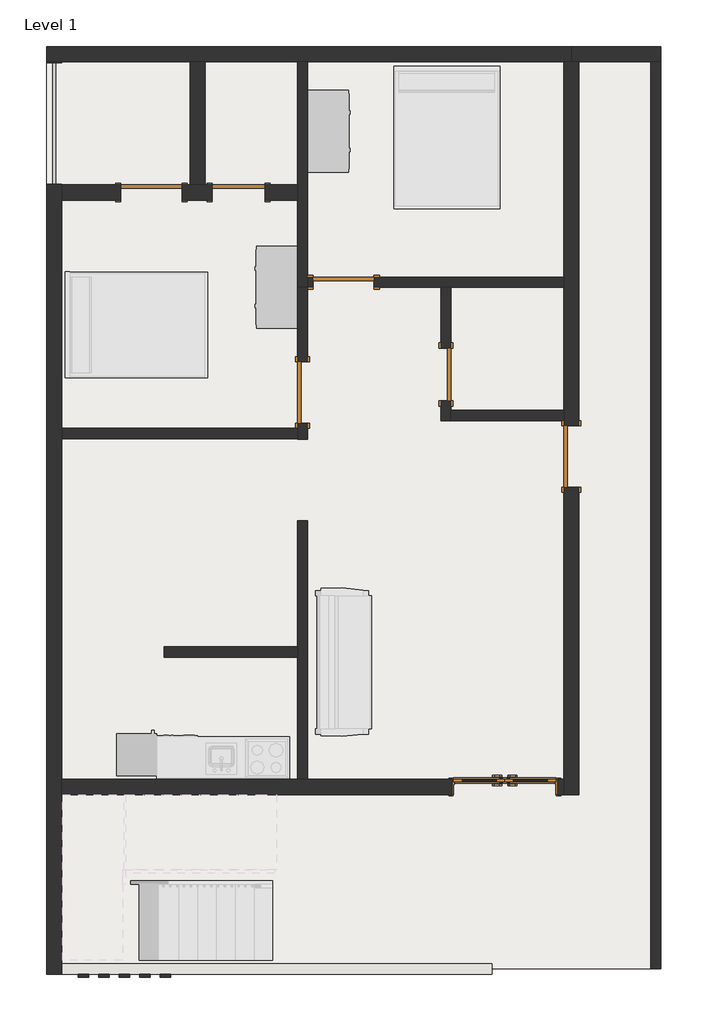
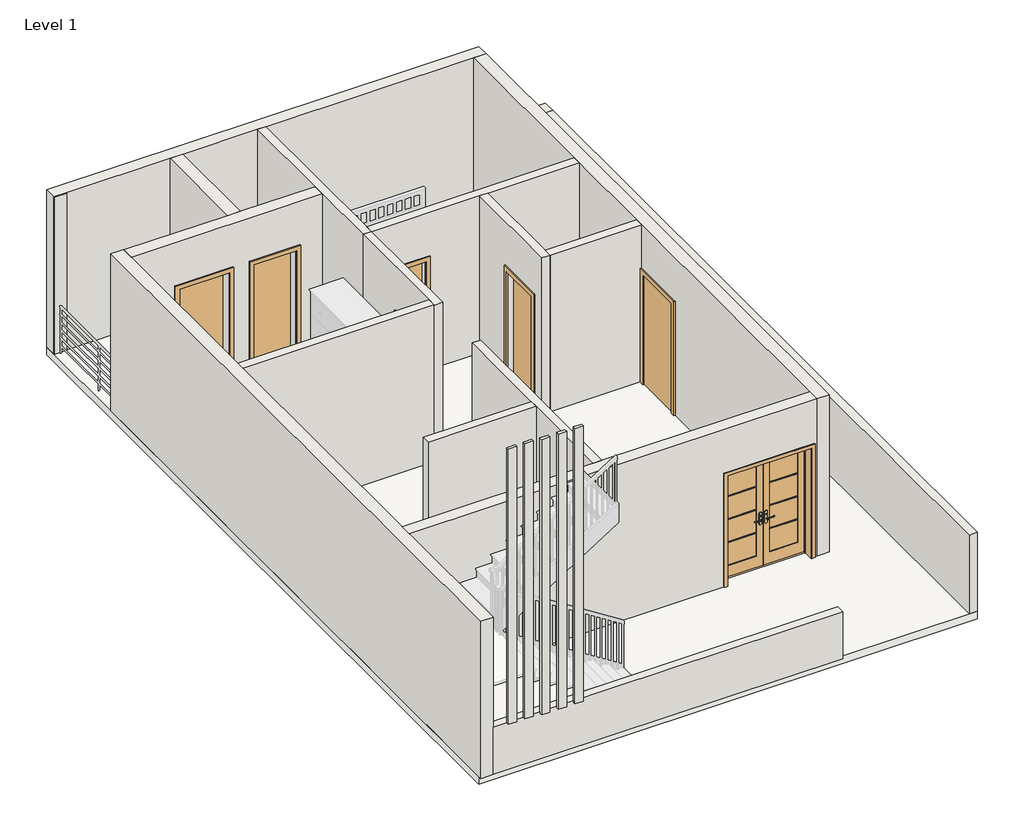
# One storey, part 1 of 2: 19 walls, 7 doors, 1 slab.
"""IFC4 building model written with IfcOpenShell, lengths in millimetres."""

from ifc_helpers import new_model, si_unit, frame, origin, origin_with_axes, place, context, project, spatial, polyline, outline, extrude, faceted_brep, transform, mapped, element, save
from components import door_014e9f54, door_486760f8, door_b804d09e, door_686f89d2, door_0ca8825f, walls_1_walls_1_4968a21e

model = new_model("IFC4")

# Units and contexts
model_context = context("Model", 3, world=origin())
ifc_project = project(units=[si_unit("LENGTHUNIT", "METRE", prefix="MILLI")], contexts=[model_context])

# Site, building, storey
site = spatial("IfcSite", under=ifc_project)
building = spatial("IfcBuilding", under=site)
storey = spatial("IfcBuildingStorey", under=building, Name="Level 1", Elevation=0.0)

# Doors
placement = place(None, origin())
door_shape = door_014e9f54(model_context)
element("IfcDoor", 1, ObjectType="Door-Exterior-Double-Full Glass-Wood_Clad : 60\" x 84\"", at=placement, inside=storey, context=model_context, shape_type="MappedRepresentation", body=[
    mapped(door_shape, transform((-4531.8683044, -1257.1141189, 0.0), x_axis=(1.0, 0.0, 0.0), y_axis=(0.0, 1.0, 0.0), z_axis=(0.0, 0.0, 1.0))),
])
door_2_shape = door_486760f8(model_context)
element("IfcDoor", 2, ObjectType="Single-Flush : 2'7\"", at=placement, inside=storey, context=model_context, shape_type="MappedRepresentation", body=[
    mapped(door_2_shape, transform((-8494.2683044, 7578.9108811, 0.0), x_axis=(-1.0, 0.0, 0.0), y_axis=(0.0, -1.0, 0.0), z_axis=(0.0, 0.0, 1.0))),
])
door_3_shape = door_b804d09e(model_context)
element("IfcDoor", 3, ObjectType="Single-Flush : 2'7\"", at=placement, inside=storey, context=model_context, shape_type="MappedRepresentation", body=[
    mapped(door_3_shape, transform((-5408.1683044, 4873.8108811, 0.0), x_axis=(0.0, -1.0, 0.0), y_axis=(1.0, 0.0, 0.0), z_axis=(0.0, 0.0, 1.0))),
])
door_4_shape = door_686f89d2(model_context)
element("IfcDoor", 4, ObjectType="Single-Flush : 36\" x 84\"", at=placement, inside=storey, context=model_context, shape_type="MappedRepresentation", body=[
    mapped(door_4_shape, transform((-6932.1683044, 6245.4108811, 0.0), x_axis=(-1.0, 0.0, 0.0), y_axis=(0.0, -1.0, 0.0), z_axis=(0.0, 0.0, 1.0))),
])
element("IfcDoor", 5, ObjectType="Single-Flush : 36\" x 84\"", at=placement, inside=storey, context=model_context, shape_type="MappedRepresentation", body=[
    mapped(door_4_shape, transform((-7541.7683044, 4607.1108811, 0.0), x_axis=(0.0, -1.0, 0.0), y_axis=(1.0, 0.0, 0.0), z_axis=(0.0, 0.0, 1.0))),
])
door_5_shape = door_0ca8825f(model_context)
element("IfcDoor", 6, ObjectType="Single-Flush : 36\" x 84\"", at=placement, inside=storey, context=model_context, shape_type="MappedRepresentation", body=[
    mapped(door_5_shape, transform((-9789.6683044, 7578.9108811, 0.0), x_axis=(1.0, 0.0, 0.0), y_axis=(0.0, 1.0, 0.0), z_axis=(0.0, 0.0, 1.0))),
])
element("IfcDoor", 7, ObjectType="Single-Flush : 36\" x 84\"", at=placement, inside=storey, context=model_context, shape_type="MappedRepresentation", body=[
    mapped(door_5_shape, transform((-3541.2683044, 3654.6108811, 0.0), x_axis=(0.0, 1.0, 0.0), y_axis=(-1.0, 0.0, 0.0), z_axis=(0.0, 0.0, 1.0))),
])

# Slab
element("IfcSlab", 8, ObjectType="6\"", at=placement, inside=storey, context=model_context, shape_type="SweptSolid", body=[
    extrude(outline(polyline([(-2207.7683044, 9750.6108811), (-2207.7683044, -3965.3891189), (-11351.7683044, -3965.3891189), (-11351.7683044, 9750.6108811), (-2207.7683044, 9750.6108811)])), frame((0.0, 0.0, -152.4), z_axis=(0.0, 0.0, 1.0), x_axis=(1.0, 0.0, 0.0)), (0.0, 0.0, 1.0), 152.4),
])

# Walls
element("IfcWall", 9, ObjectType="6\"", at=placement, inside=storey, context=model_context, shape_type="SweptSolid", body=[
    extrude(outline(polyline([(-2360.1683044, -3965.3891189), (-2360.1683044, 9522.0108811), (-2207.7683044, 9522.0108811), (-2207.7683044, -3965.3891189), (-2360.1683044, -3965.3891189)])), origin_with_axes(), (0.0, 0.0, 1.0), 1524.0),
])
element("IfcWall", 10, ObjectType="6\"", at=placement, inside=storey, context=model_context, shape_type="SweptSolid", body=[
    extrude(outline(polyline([(-11123.1683044, -3889.1891189), (-4722.3683044, -3889.1891189), (-4722.3683044, -4041.5891189), (-11123.1683044, -4041.5891189), (-11123.1683044, -3889.1891189)])), origin_with_axes(), (0.0, 0.0, 1.0), 914.4),
])
element("IfcWall", 11, ObjectType="6\" 2", at=placement, inside=storey, context=model_context, shape_type="Brep", body=[
    faceted_brep([(-7617.9683044, 9522.0108811, 0.0), (-7617.9683044, 7693.2108811, 0.0), (-7617.9683044, 7464.6108811, 0.0), (-7617.9683044, 6169.2108811, 0.0), (-7617.9683044, 6169.2108811, 3048.0), (-7617.9683044, 7464.6108811, 3048.0), (-7617.9683044, 7693.2108811, 3048.0), (-7617.9683044, 9522.0108811, 3048.0), (-7465.5683044, 9522.0108811, 0.0), (-7465.5683044, 9522.0108811, 3048.0), (-7465.5683044, 6321.6108811, 3048.0), (-7465.5683044, 6169.2108811, 3048.0), (-7465.5683044, 6169.2108811, 0.0), (-7465.5683044, 6321.6108811, 0.0)], [[[0, 1, 2, 3, 4, 5, 6, 7]], [[8, 9, 10, 11, 12, 13]], [[3, 2, 1, 0, 8, 13, 12]], [[7, 6, 5, 4, 11, 10, 9]], [[0, 7, 9, 8]], [[4, 3, 12, 11]]]),
])
element("IfcWall", 12, ObjectType="6\" 2", at=placement, inside=storey, context=model_context, shape_type="Brep", body=[
    faceted_brep([(-7465.5683044, 6169.2108811, 0.0), (-7389.3683044, 6169.2108811, 0.0), (-7389.3683044, 6169.2108811, 2133.6), (-6474.9683044, 6169.2108811, 2133.6), (-6474.9683044, 6169.2108811, 0.0), (-5484.3683044, 6169.2108811, 0.0), (-5331.9683044, 6169.2108811, 0.0), (-3655.5683044, 6169.2108811, 0.0), (-3655.5683044, 6169.2108811, 3048.0), (-5331.9683044, 6169.2108811, 3048.0), (-5484.3683044, 6169.2108811, 3048.0), (-7465.5683044, 6169.2108811, 3048.0), (-7389.3683044, 6321.6108811, 2133.6), (-7389.3683044, 6321.6108811, 0.0), (-7465.5683044, 6321.6108811, 0.0), (-7465.5683044, 6321.6108811, 3048.0), (-3655.5683044, 6321.6108811, 3048.0), (-3655.5683044, 6321.6108811, 0.0), (-6474.9683044, 6321.6108811, 0.0), (-6474.9683044, 6321.6108811, 2133.6)], [[[0, 1, 2, 3, 4, 5, 6, 7, 8, 9, 10, 11]], [[12, 13, 14, 15, 16, 17, 18, 19]], [[18, 17, 7, 6, 5, 4]], [[14, 13, 1, 0]], [[11, 10, 9, 8, 16, 15]], [[0, 11, 15, 14]], [[8, 7, 17, 16]], [[2, 1, 13, 12]], [[3, 2, 12, 19]], [[4, 3, 19, 18]]]),
])
element("IfcWall", 13, ObjectType="6\" 2", at=placement, inside=storey, context=model_context, shape_type="Brep", body=[
    faceted_brep([(-7617.9683044, 4149.9108811, 2133.6), (-7617.9683044, 4149.9108811, 0.0), (-7617.9683044, 4073.7108811, 0.0), (-7617.9683044, 3921.3108811, 0.0), (-7617.9683044, 3908.6108811, 0.0), (-7617.9683044, 3908.6108811, 3048.0), (-7617.9683044, 3921.3108811, 3048.0), (-7617.9683044, 4073.7108811, 3048.0), (-7617.9683044, 6169.2108811, 3048.0), (-7617.9683044, 6169.2108811, 0.0), (-7617.9683044, 5064.3108811, 0.0), (-7617.9683044, 5064.3108811, 2133.6), (-7465.5683044, 3908.6108811, 0.0), (-7465.5683044, 4149.9108811, 0.0), (-7465.5683044, 4149.9108811, 2133.6), (-7465.5683044, 5064.3108811, 2133.6), (-7465.5683044, 5064.3108811, 0.0), (-7465.5683044, 6169.2108811, 0.0), (-7465.5683044, 6169.2108811, 3048.0), (-7465.5683044, 3908.6108811, 3048.0)], [[[0, 1, 2, 3, 4, 5, 6, 7, 8, 9, 10, 11]], [[12, 13, 14, 15, 16, 17, 18, 19]], [[10, 9, 17, 16]], [[4, 3, 2, 1, 13, 12]], [[5, 4, 12, 19]], [[8, 7, 6, 5, 19, 18]], [[9, 8, 18, 17]], [[14, 13, 1, 0]], [[15, 14, 0, 11]], [[16, 15, 11, 10]]]),
])
element("IfcWall", 14, ObjectType="6\" 2", at=placement, inside=storey, context=model_context, shape_type="SweptSolid", body=[
    extrude(outline(polyline([(-7617.9683044, 3921.3108811), (-11123.1683044, 3921.3108811), (-11123.1683044, 4073.7108811), (-7617.9683044, 4073.7108811), (-7617.9683044, 3921.3108811)])), origin_with_axes(), (0.0, 0.0, 1.0), 3048.0),
])
element("IfcWall", 15, ObjectType="6\" 2", at=placement, inside=storey, context=model_context, shape_type="SweptSolid", body=[
    extrude(outline(polyline([(-9599.1683044, 822.5108811), (-7617.9683044, 822.5108811), (-7617.9683044, 670.1108811), (-9599.1683044, 670.1108811), (-9599.1683044, 822.5108811)])), origin_with_axes(), (0.0, 0.0, 1.0), 3048.0),
])
element("IfcWall", 16, ObjectType="6\" 2", at=placement, inside=storey, context=model_context, shape_type="Brep", body=[
    faceted_brep([(-5484.3683044, 4480.1108811, 2133.6), (-5484.3683044, 4480.1108811, 0.0), (-5484.3683044, 4188.0108811, 0.0), (-5484.3683044, 4188.0108811, 3048.0), (-5484.3683044, 6169.2108811, 3048.0), (-5484.3683044, 6169.2108811, 0.0), (-5484.3683044, 5267.5108811, 0.0), (-5484.3683044, 5267.5108811, 2133.6), (-5331.9683044, 4188.0108811, 0.0), (-5331.9683044, 4480.1108811, 0.0), (-5331.9683044, 4480.1108811, 2133.6), (-5331.9683044, 5267.5108811, 2133.6), (-5331.9683044, 5267.5108811, 0.0), (-5331.9683044, 6169.2108811, 0.0), (-5331.9683044, 6169.2108811, 3048.0), (-5331.9683044, 4340.4108811, 3048.0), (-5331.9683044, 4188.0108811, 3048.0), (-5331.9683044, 4188.0108811, 13.8133607)], [[[0, 1, 2, 3, 4, 5, 6, 7]], [[8, 9, 10, 11, 12, 13, 14, 15, 16, 17]], [[6, 5, 13, 12]], [[2, 1, 9, 8]], [[4, 3, 16, 15, 14]], [[5, 4, 14, 13]], [[3, 2, 8, 17, 16]], [[10, 9, 1, 0]], [[11, 10, 0, 7]], [[12, 11, 7, 6]]]),
])
element("IfcWall", 17, ObjectType="6\" 2", at=placement, inside=storey, context=model_context, shape_type="SweptSolid", body=[
    extrude(outline(polyline([(-3655.5683044, 4188.0108811), (-5331.9683044, 4188.0108811), (-5331.9683044, 4340.4108811), (-3655.5683044, 4340.4108811), (-3655.5683044, 4188.0108811)])), frame((0.0, 0.0, 13.8133607), z_axis=(0.0, 0.0, 1.0), x_axis=(1.0, 0.0, 0.0)), (0.0, 0.0, 1.0), 3034.1866393),
])
element("IfcWall", 18, ObjectType="6\" 2", at=placement, inside=storey, context=model_context, shape_type="Brep", body=[
    faceted_brep([(-7617.9683044, 2702.1108811, 0.0), (-7617.9683044, 822.5108811, 0.0), (-7617.9683044, 670.1108811, 0.0), (-7617.9683044, -1145.9891189, 0.0), (-7617.9683044, -1145.9891189, 3048.0), (-7617.9683044, 670.1108811, 3048.0), (-7617.9683044, 822.5108811, 3048.0), (-7617.9683044, 2702.1108811, 3048.0), (-7465.5683044, 2702.1108811, 0.0), (-7465.5683044, 2702.1108811, 3048.0), (-7465.5683044, -1145.9891189, 3048.0), (-7465.5683044, -1145.9891189, 0.0)], [[[0, 1, 2, 3, 4, 5, 6, 7]], [[8, 9, 10, 11]], [[3, 2, 1, 0, 8, 11]], [[7, 6, 5, 4, 10, 9]], [[0, 7, 9, 8]], [[4, 3, 11, 10]]]),
])
element("IfcWall", 19, ObjectType="9\"", at=placement, inside=storey, context=model_context, shape_type="Brep", body=[
    faceted_brep([(-11351.7683044, 9522.0108811, 0.0), (-11123.1683044, 9522.0108811, 0.0), (-9218.1683044, 9522.0108811, 0.0), (-8989.5683044, 9522.0108811, 0.0), (-7617.9683044, 9522.0108811, 0.0), (-7465.5683044, 9522.0108811, 0.0), (-3655.5683044, 9522.0108811, 0.0), (-3541.2683044, 9522.0108811, 0.0), (-3541.2683044, 9522.0108811, 1524.0), (-3426.9683044, 9522.0108811, 1524.0), (-3426.9683044, 9522.0108811, 3048.0), (-3655.5683044, 9522.0108811, 3048.0), (-7465.5683044, 9522.0108811, 3048.0), (-7617.9683044, 9522.0108811, 3048.0), (-8989.5683044, 9522.0108811, 3048.0), (-9218.1683044, 9522.0108811, 3048.0), (-11123.1683044, 9522.0108811, 3048.0), (-11351.7683044, 9522.0108811, 3048.0), (-11351.7683044, 9750.6108811, 0.0), (-11351.7683044, 9750.6108811, 3048.0), (-3426.9683044, 9750.6108811, 3048.0), (-3426.9683044, 9750.6108811, 1524.0), (-3541.2683044, 9750.6108811, 1524.0), (-3541.2683044, 9750.6108811, 0.0)], [[[0, 1, 2, 3, 4, 5, 6, 7, 8, 9, 10, 11, 12, 13, 14, 15, 16, 17]], [[18, 19, 20, 21, 22, 23]], [[7, 6, 5, 4, 3, 2, 1, 0, 18, 23]], [[17, 16, 15, 14, 13, 12, 11, 10, 20, 19]], [[0, 17, 19, 18]], [[8, 7, 23, 22]], [[21, 9, 8, 22]], [[10, 9, 21, 20]]]),
])
element("IfcWall", 20, ObjectType="9\"", at=placement, inside=storey, context=model_context, shape_type="Brep", body=[
    faceted_brep([(-11123.1683044, -4041.5891189, 0.0), (-11123.1683044, -3889.1891189, 0.0), (-11123.1683044, -1374.5891189, 0.0), (-11123.1683044, -1145.9891189, 0.0), (-11123.1683044, 3921.3108811, 0.0), (-11123.1683044, 4073.7108811, 0.0), (-11123.1683044, 7464.6108811, 0.0), (-11123.1683044, 7693.2108811, 0.0), (-11123.1683044, 7705.9108811, 0.0), (-11123.1683044, 7705.9108811, 3048.0), (-11123.1683044, 7693.2108811, 3048.0), (-11123.1683044, 7464.6108811, 3048.0), (-11123.1683044, 4073.7108811, 3048.0), (-11123.1683044, 3921.3108811, 3048.0), (-11123.1683044, -1145.9891189, 3048.0), (-11123.1683044, -1374.5891189, 3048.0), (-11123.1683044, -4041.5891189, 3048.0), (-11123.1683044, -4041.5891189, 914.4), (-11351.7683044, -4041.5891189, 0.0), (-11351.7683044, -4041.5891189, 3048.0), (-11351.7683044, 7705.9108811, 3048.0), (-11351.7683044, 7705.9108811, 0.0)], [[[0, 1, 2, 3, 4, 5, 6, 7, 8, 9, 10, 11, 12, 13, 14, 15, 16, 17]], [[18, 19, 20, 21]], [[8, 7, 6, 5, 4, 3, 2, 1, 0, 18, 21]], [[9, 8, 21, 20]], [[16, 15, 14, 13, 12, 11, 10, 9, 20, 19]], [[0, 17, 16, 19, 18]]]),
])
element("IfcWall", 21, ObjectType="9\"", at=placement, inside=storey, context=model_context, shape_type="Brep", body=[
    faceted_brep([(-3655.5683044, -1374.5891189, 3048.0), (-3655.5683044, -1145.9891189, 3048.0), (-3655.5683044, 4188.0108811, 3048.0), (-3655.5683044, 4340.4108811, 3048.0), (-3655.5683044, 6169.2108811, 3048.0), (-3655.5683044, 6321.6108811, 3048.0), (-3655.5683044, 9522.0108811, 3048.0), (-3655.5683044, 9522.0108811, 0.0), (-3655.5683044, 6321.6108811, 0.0), (-3655.5683044, 6169.2108811, 0.0), (-3655.5683044, 4111.8108811, 0.0), (-3655.5683044, 4111.8108811, 2133.6), (-3655.5683044, 3197.4108811, 2133.6), (-3655.5683044, 3197.4108811, 0.0), (-3655.5683044, -1145.9891189, 0.0), (-3655.5683044, -1374.5891189, 0.0), (-3426.9683044, 9522.0108811, 3048.0), (-3426.9683044, -1374.5891189, 3048.0), (-3426.9683044, -1374.5891189, 0.0), (-3426.9683044, 3197.4108811, 0.0), (-3426.9683044, 3197.4108811, 2133.6), (-3426.9683044, 4111.8108811, 2133.6), (-3426.9683044, 4111.8108811, 0.0), (-3426.9683044, 9522.0108811, 0.0), (-3426.9683044, 9522.0108811, 1524.0), (-3541.2683044, 9522.0108811, 0.0)], [[[0, 1, 2, 3, 4, 5, 6, 7, 8, 9, 10, 11, 12, 13, 14, 15]], [[16, 17, 18, 19, 20, 21, 22, 23, 24]], [[18, 15, 14, 13, 19]], [[7, 25, 23, 22, 10, 9, 8]], [[6, 5, 4, 3, 2, 1, 0, 17, 16]], [[0, 15, 18, 17]], [[23, 25, 7, 6, 16, 24]], [[21, 11, 10, 22]], [[11, 21, 20, 12]], [[12, 20, 19, 13]]]),
])
element("IfcWall", 22, ObjectType="9\"", at=placement, inside=storey, context=model_context, shape_type="Brep", body=[
    faceted_brep([(-11123.1683044, -1145.9891189, 3048.0), (-7617.9683044, -1145.9891189, 3048.0), (-7465.5683044, -1145.9891189, 3048.0), (-3655.5683044, -1145.9891189, 3048.0), (-3655.5683044, -1145.9891189, 0.0), (-3744.4683044, -1145.9891189, 0.0), (-3744.4683044, -1145.9891189, 2159.0), (-5319.2683044, -1145.9891189, 2159.0), (-5319.2683044, -1145.9891189, 0.0), (-7465.5683044, -1145.9891189, 0.0), (-7617.9683044, -1145.9891189, 0.0), (-11123.1683044, -1145.9891189, 0.0), (-3655.5683044, -1374.5891189, 3048.0), (-11123.1683044, -1374.5891189, 3048.0), (-11123.1683044, -1374.5891189, 0.0), (-5319.2683044, -1374.5891189, 0.0), (-5319.2683044, -1374.5891189, 2159.0), (-3744.4683044, -1374.5891189, 2159.0), (-3744.4683044, -1374.5891189, 0.0), (-3655.5683044, -1374.5891189, 0.0)], [[[0, 1, 2, 3, 4, 5, 6, 7, 8, 9, 10, 11]], [[12, 13, 14, 15, 16, 17, 18, 19]], [[4, 19, 18, 5]], [[14, 11, 10, 9, 8, 15]], [[3, 2, 1, 0, 13, 12]], [[4, 3, 12, 19]], [[0, 11, 14, 13]], [[17, 6, 5, 18]], [[6, 17, 16, 7]], [[7, 16, 15, 8]]]),
])
element("IfcWall", 23, ObjectType="9\"", at=placement, inside=storey, context=model_context, shape_type="Brep", body=[
    faceted_brep([(-9332.4683044, 7464.6108811, 0.0), (-8887.9683044, 7464.6108811, 0.0), (-8887.9683044, 7464.6108811, 2133.6), (-8100.5683044, 7464.6108811, 2133.6), (-8100.5683044, 7464.6108811, 0.0), (-7617.9683044, 7464.6108811, 0.0), (-7617.9683044, 7464.6108811, 3048.0), (-11123.1683044, 7464.6108811, 3048.0), (-11123.1683044, 7464.6108811, 0.0), (-10246.8683044, 7464.6108811, 0.0), (-10246.8683044, 7464.6108811, 2133.6), (-9332.4683044, 7464.6108811, 2133.6), (-8887.9683044, 7693.2108811, 2133.6), (-8887.9683044, 7693.2108811, 0.0), (-8989.5683044, 7693.2108811, 0.0), (-9218.1683044, 7693.2108811, 0.0), (-9332.4683044, 7693.2108811, 0.0), (-9332.4683044, 7693.2108811, 2133.6), (-10246.8683044, 7693.2108811, 2133.6), (-10246.8683044, 7693.2108811, 0.0), (-11123.1683044, 7693.2108811, 0.0), (-11123.1683044, 7693.2108811, 3048.0), (-9218.1683044, 7693.2108811, 3048.0), (-8989.5683044, 7693.2108811, 3048.0), (-7617.9683044, 7693.2108811, 3048.0), (-7617.9683044, 7693.2108811, 0.0), (-8100.5683044, 7693.2108811, 0.0), (-8100.5683044, 7693.2108811, 2133.6)], [[[0, 1, 2, 3, 4, 5, 6, 7, 8, 9, 10, 11]], [[12, 13, 14, 15, 16, 17, 18, 19, 20, 21, 22, 23, 24, 25, 26, 27]], [[9, 8, 20, 19]], [[26, 25, 5, 4]], [[16, 15, 14, 13, 1, 0]], [[7, 6, 24, 23, 22, 21]], [[8, 7, 21, 20]], [[17, 16, 0, 11]], [[18, 17, 11, 10]], [[19, 18, 10, 9]], [[2, 1, 13, 12]], [[3, 2, 12, 27]], [[4, 3, 27, 26]], [[6, 5, 25, 24]]]),
])
element("IfcWall", 24, ObjectType="9\"", at=placement, inside=storey, context=model_context, shape_type="SweptSolid", body=[
    extrude(outline(polyline([(-8989.5683044, 9522.0108811), (-8989.5683044, 7693.2108811), (-9218.1683044, 7693.2108811), (-9218.1683044, 9522.0108811), (-8989.5683044, 9522.0108811)])), origin_with_axes(), (0.0, 0.0, 1.0), 3048.0),
])
element("IfcWall", 25, ObjectType="9\"", at=placement, inside=storey, context=model_context, shape_type="Brep", body=[
    faceted_brep([(-3541.2683044, 9522.0108811, 0.0), (-3426.9683044, 9522.0108811, 0.0), (-2360.1683044, 9522.0108811, 0.0), (-2207.7683044, 9522.0108811, 0.0), (-2207.7683044, 9522.0108811, 1524.0), (-2360.1683044, 9522.0108811, 1524.0), (-3426.9683044, 9522.0108811, 1524.0), (-3541.2683044, 9522.0108811, 1524.0), (-3541.2683044, 9750.6108811, 0.0), (-3541.2683044, 9750.6108811, 1524.0), (-3426.9683044, 9750.6108811, 1524.0), (-2207.7683044, 9750.6108811, 1524.0), (-2207.7683044, 9750.6108811, 0.0)], [[[0, 1, 2, 3, 4, 5, 6, 7]], [[8, 9, 10, 11, 12]], [[3, 2, 1, 0, 8, 12]], [[7, 6, 5, 4, 11, 10, 9]], [[0, 7, 9, 8]], [[4, 3, 12, 11]]]),
])
element("IfcWall", 26, ObjectType="9\"", at=placement, inside=storey, context=model_context, shape_type="SweptSolid", body=[
    extrude(outline(polyline([(-11123.1683044, 9522.0108811), (-11123.1683044, 9509.3108811), (-11351.7683044, 9509.3108811), (-11351.7683044, 9522.0108811), (-11123.1683044, 9522.0108811)])), origin_with_axes(), (0.0, 0.0, 1.0), 3048.0),
])
walls_1_walls_1_shape = walls_1_walls_1_4968a21e(model_context)
element("IfcWall", 27, ObjectType="Walls 1 : Walls 1", at=placement, inside=storey, context=model_context, shape_type="MappedRepresentation", body=[
    mapped(walls_1_walls_1_shape, transform((0.0, 0.0, 0.0), x_axis=(1.0, 0.0, 0.0), y_axis=(0.0, 1.0, 0.0), z_axis=(0.0, 0.0, 1.0))),
])

save(model, "model.ifc")

# Revit data of these elements
# Type "Door-Exterior-Double-Full Glass-Wood_Clad : 60\" x 84\""
#   Type Mark = "9"
#   Assembly Code = "B2030100"
#   Analytic Construction = "French door, wood frame with double glass"
#   Top Rail = 0' - 4 11/16"
#   Threshold Offset [instance default] = 0' - 0 1/2"
#   Thickness = 0' - 1 3/8"
#   Thermal Resistance (R) = 1.9158 (h·ft²·°F)/BTU
#   Swing Angle [instance default] = 90.00°
#   Stiles = 0' - 4 3/4"
#   Rough Width = 5' - 2"
#   Rough Height = 7' - 1"
#   Panel Width = 2' - 6"
#   Door Offset [instance default] = 0' - 0"
#   Height = 7' - 0"
#   Width = 5' - 0"
#   Heat Transfer Coefficient (U) = 0.5220 BTU/(h·ft²·°F)
#   Bottom Rail = 0' - 9 1/8"
#   Exterior Trim [instance default] = yes
#   Threshold [instance default] = yes
#   Show Grill [instance default] = yes
#   Function = 1
#   Trim Material = Cherry
#   Threshold Material = Cherry
#   Panel Material = Cherry
#   Glazing = Glass
#   Frame Material = Cherry
#   Door Handle Material = Aluminum
#   Visual Light Transmittance = 0
#   Solar Heat Gain Coefficient = 0
#   Wall Closure = (empty or 0)
#   Construction Type = (empty or 0)
# Type "Single-Flush : 2'7\""
#   Type Mark = "8"
#   Construction Type Id = "MDOOR"
#   Assembly Code = "C1020"
#   Analytic Construction = "Metal"
#   Thickness = 0' - 2"
#   Heat Transfer Coefficient (U) = 0.651978 BTU/(h·ft²·°F)
#   Height = 7' - 0"
#   Trim Projection Ext = 0' - 1"
#   Trim Projection Int = 0' - 1"
#   Trim Width = 0' - 3"
#   Width = 2' - 7"
#   Define Thermal Properties by = 1
#   Door Material = Door - Panel
#   Frame Material = Door - Frame
#   Visual Light Transmittance = 0
#   Solar Heat Gain Coefficient = 0
#   Function = (empty or 0)
#   Wall Closure = (empty or 0)
# Type "Single-Flush : 36\" x 84\""
#   Type Mark = "1"
#   Construction Type Id = "MDOOR"
#   Assembly Code = "C1020"
#   Analytic Construction = "Metal"
#   Thickness = 0' - 2"
#   Heat Transfer Coefficient (U) = 0.651978 BTU/(h·ft²·°F)
#   Height = 7' - 0"
#   Trim Projection Ext = 0' - 1"
#   Trim Projection Int = 0' - 1"
#   Trim Width = 0' - 3"
#   Width = 3' - 0"
#   Define Thermal Properties by = 1
#   Door Material = Door - Panel
#   Frame Material = Door - Frame
#   Visual Light Transmittance = 0
#   Solar Heat Gain Coefficient = 0
#   Function = (empty or 0)
#   Wall Closure = (empty or 0)
# Type "6\""
#   Assembly Code = "B1010"
#   Function = 0
#   Layers, outside or top first: 0' - 6" "floor" (function 1)
# Type "6\""
#   Assembly Code = "B2010"
#   Layers, outside or top first: 0' - 6" "ext wall" (function 1)
# Type "6\" 2"
#   Assembly Code = "B2010"
#   Layers, outside or top first: 0' - 6" no material (function 1)
# Type "9\""
#   Assembly Code = "B2010"
#   Layers, outside or top first: 0' - 9" "ext wall" (function 1)
# Element 1 (IfcDoor, "Door-Exterior-Double-Full Glass-Wood_Clad : 60\" x 84\"")
#   Threshold Offset = 0' - 0 1/2"
#   Swing Angle = 90.00°
#   Door Offset = 0' - 0"
#   Threshold = yes
#   Show Grill = yes
#   Exterior Trim = yes
#   Phase Created = New Construction
#   Materials on its faces: "Cherry", "Aluminum", "Glass"
# Elements 2, 3 (IfcDoor, "Single-Flush : 2'7\"")
#   Phase Created = New Construction
#   Materials on its faces: "Door - Frame", "Door - Panel"
# Elements 4, 5, 6, 7 (IfcDoor, "Single-Flush : 36\" x 84\"")
#   Phase Created = New Construction
#   Materials on its faces: "Door - Frame", "Door - Panel"
# Element 8 (IfcSlab, "6\"")
#   Height Offset From Level = 0' - 0"
#   Phase Created = New Construction
#   Materials on its faces: "floor"
# Element 9 (IfcWall, "6\"")
#   Top Offset = 0' - 0"
#   Base Offset = 0' - 0"
#   Unconnected Height = 5' - 0"
#   wall height = 5' - 0"
#   Phase Created = New Construction
#   Base Constraint = Level 1
#   Materials on its faces: "ext wall"
# Element 10 (IfcWall, "6\"")
#   Top Offset = 0' - 0"
#   Base Offset = 0' - 0"
#   Unconnected Height = 3' - 0"
#   wall height = 3' - 0"
#   Phase Created = New Construction
#   Base Constraint = Level 1
#   Materials on its faces: "ext wall"
# Elements 11, 12, 13, 14, 15, 16, 18 (IfcWall, "6\" 2")
#   Top Offset = 0' - 0"
#   Base Offset = 0' - 0"
#   Unconnected Height = 10' - 0"
#   wall height = 10' - 0"
#   Phase Created = New Construction
#   Base Constraint = Level 1
#   Materials on its faces: "Default Wall"
# Element 17 (IfcWall, "6\" 2")
#   built-in parameter 1001111 = 0' - 0.54383"
#   Top Offset = 0' - 0"
#   Base Offset = 0' - 0.54383"
#   Unconnected Height = 9' - 11.45617"
#   wall height = 9' - 11.45617"
#   Phase Created = New Construction
#   Base Constraint = Level 1
#   Materials on its faces: "Default Wall"
# Elements 19, 20, 21, 22, 23, 24, 26 (IfcWall, "9\"")
#   Top Offset = 0' - 0"
#   Base Offset = 0' - 0"
#   Unconnected Height = 10' - 0"
#   wall height = 10' - 0"
#   Phase Created = New Construction
#   Base Constraint = Level 1
#   Materials on its faces: "ext wall"
# Element 25 (IfcWall, "9\"")
#   Top Offset = 0' - 0"
#   Base Offset = 0' - 0"
#   Unconnected Height = 5' - 0"
#   wall height = 5' - 0"
#   Phase Created = New Construction
#   Base Constraint = Level 1
#   Materials on its faces: "ext wall"
# Element 27 (IfcWall, "Walls 1 : Walls 1")
#   Phase Created = New Construction
#   Materials on its faces: "DESIGN"
# Materials
#   "Cherry": class "Wood", colour RGB 226 177 128, transparency 0, Description = "Prunus Serotina", Cost = 0
#   "Glass": class "Glass", colour RGB 0 128 192, transparency 0.75, Description = "Soda Lime Glass", Cost = 0
#   "Aluminum": class "Metal", colour RGB 247 247 247, transparency 0, Description = "Aluminum 6061", Cost = 0
#   "Door - Panel": class "Wood", colour RGB 210 159 95, transparency 0
#   "Door - Frame": colour RGB 118 70 51, transparency 0
#   "floor": class "Generic", colour RGB 146 137 125, transparency 0, Cost = 0
#   "ext wall": class "Generic", colour RGB 230 213 172, transparency 0, Cost = 0
#   "Default Wall": colour RGB 128 128 128, transparency 0
#   "DESIGN": class "Generic", colour RGB 255 214 0, transparency 0, Cost = 0
